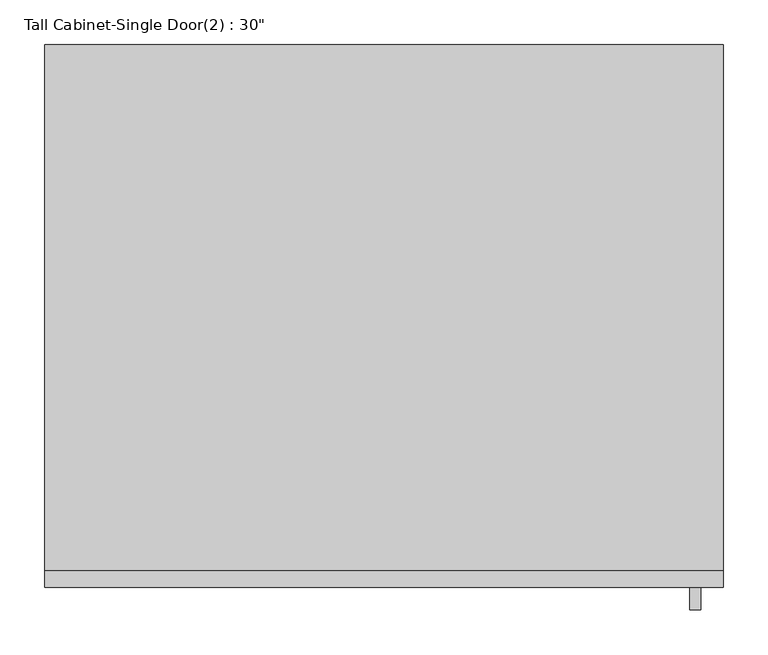
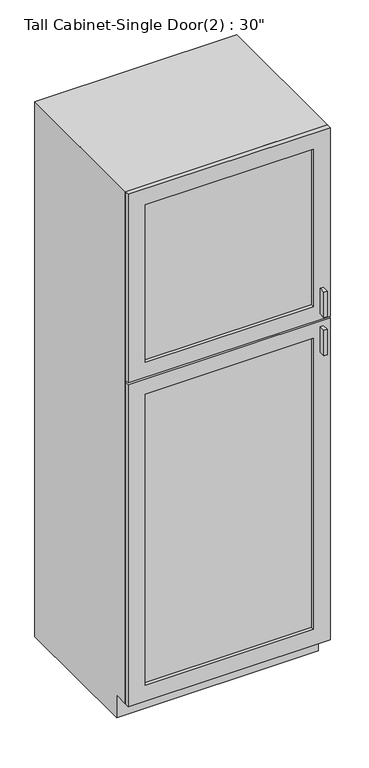
"""IFC4 building model written with IfcOpenShell, lengths in millimetres: furniture geometry."""

from ifc_helpers import new_model, si_unit, frame, origin, place, context, project, spatial, polyline, outline, extrude, faceted_brep, source, transform, mapped, element, save


def furniture_7f1a6afb(model_context):
    return source(origin(), model_context, "Body", "SolidModel", [
        faceted_brep([(399.7377049, -590.55, 90.4875), (399.7377049, -590.55, 2133.6), (-362.2622951, -590.55, 2133.6), (-362.2622951, -590.55, 90.4875), (380.6877049, -590.55, 2114.55), (380.6877049, -590.55, 109.5375), (-343.2122951, -590.55, 109.5375), (-343.2122951, -590.55, 2114.55), (-362.2622951, 0.0, 2133.6), (399.7377049, 0.0, 2133.6), (399.7377049, 0.0, 0.0), (-362.2622951, 0.0, 0.0), (399.7377049, -533.4, 90.4875), (399.7377049, -533.4, 0.0), (-362.2622951, -533.4, 0.0), (-362.2622951, -533.4, 90.4875), (380.6877049, -19.05, 2114.55), (380.6877049, -19.05, 109.5375), (-343.2122951, -19.05, 109.5375), (-343.2122951, -19.05, 2114.55)], [[[0, 1, 2, 3], [4, 5, 6, 7]], [[8, 9, 10, 11]], [[1, 0, 12, 13, 10, 9]], [[2, 1, 9, 8]], [[3, 2, 8, 11, 14, 15]], [[0, 3, 15, 12]], [[5, 4, 16, 17]], [[6, 5, 17, 18]], [[7, 6, 18, 19]], [[4, 7, 19, 16]], [[10, 13, 14, 11]], [[14, 13, 12, 15]], [[17, 16, 19, 18]]]),
        extrude(outline(polyline([(374.3377049, -635.0), (361.8054733, -635.0), (361.8054733, -609.6), (374.3377049, -609.6), (374.3377049, -635.0)])), frame((0.0, 0.0, 1403.5480367), z_axis=(0.0, 0.0, 1.0), x_axis=(1.0, 0.0, 0.0)), (0.0, 0.0, 1.0), 101.6),
        extrude(outline(polyline([(374.3377049, -635.0), (361.8054733, -635.0), (361.8054733, -609.6), (374.3377049, -609.6), (374.3377049, -635.0)])), frame((0.0, 0.0, 1251.1480367), z_axis=(0.0, 0.0, 1.0), x_axis=(1.0, 0.0, 0.0)), (0.0, 0.0, 1.0), 101.6),
        extrude(outline(polyline([(336.2377049, -596.9), (-298.7622951, -596.9), (-298.7622951, -590.55), (336.2377049, -590.55), (336.2377049, -596.9)])), frame((0.0, 0.0, 1441.6480367), z_axis=(0.0, 0.0, 1.0), x_axis=(1.0, 0.0, 0.0)), (0.0, 0.0, 1.0), 628.4519633),
        extrude(outline(polyline([(336.2377049, -596.9), (-298.7622951, -596.9), (-298.7622951, -590.55), (336.2377049, -590.55), (336.2377049, -596.9)])), frame((0.0, 0.0, 153.9875), z_axis=(0.0, 0.0, 1.0), x_axis=(1.0, 0.0, 0.0)), (0.0, 0.0, 1.0), 1160.6605367),
        extrude(outline(polyline([(2133.6, 399.7377049), (2133.6, -362.2622951), (1381.3230367, -362.2622951), (1381.3230367, 399.7377049), (2133.6, 399.7377049)]), holes=[polyline([(2070.1, 336.2377049), (1441.6480367, 336.2377049), (1441.6480367, -298.7622951), (2070.1, -298.7622951), (2070.1, 336.2377049)])]), frame((0.0, -609.6, 0.0), z_axis=(0.0, 1.0, 0.0), x_axis=(0.0, 0.0, 1.0)), (0.0, 0.0, 1.0), 19.05),
        extrude(outline(polyline([(90.4875, 399.7377049), (1374.9730367, 399.7377049), (1374.9730367, -362.2622951), (90.4875, -362.2622951), (90.4875, 399.7377049)]), holes=[polyline([(1314.6480367, 336.2377049), (153.9875, 336.2377049), (153.9875, -298.7622951), (1314.6480367, -298.7622951), (1314.6480367, 336.2377049)])]), frame((0.0, -609.6, 0.0), z_axis=(0.0, 1.0, 0.0), x_axis=(0.0, 0.0, 1.0)), (0.0, 0.0, 1.0), 19.05),
    ])


if __name__ == "__main__":
    model = new_model("IFC4")
    model_context = context("Model", 3, world=origin())
    ifc_project = project(units=[si_unit("LENGTHUNIT", "METRE", prefix="MILLI")], contexts=[model_context])
    site = spatial("IfcSite", under=ifc_project)
    building = spatial("IfcBuilding", under=site)
    placement = place(None, origin())
    furniture_shape = furniture_7f1a6afb(model_context)
    element("IfcFurniture", 1, ObjectType="Tall Cabinet-Single Door(2) : 30\"", at=placement, inside=building, context=model_context, shape_type="MappedRepresentation", body=[
        mapped(furniture_shape, transform((0.0, 0.0, 0.0), x_axis=(1.0, 0.0, 0.0), y_axis=(0.0, 1.0, 0.0), z_axis=(0.0, 0.0, 1.0))),
    ])
    save(model, "model.ifc")

# Revit data of these elements
# Type "Tall Cabinet-Single Door(2) : 30\""
#   Assembly Code = "C1030410"
#   Depth = 2' - 0"
#   Height = 7' - 0"
#   Toe Depth = 0' - 3"
#   Toe Height = 0' - 3 1/2"
#   Width = 2' - 6"
#   Cabinet Material = none
#   Door/Drawer Material = none
#   Handle Material = Cabinets - Handles
#   Panel Material = none
#   Default Elevation = 0
# Element 1 (IfcFurniture, "Tall Cabinet-Single Door(2) : 30\"")
#   Materials on its faces: "Cabinets", "Cabinets - Handles"
# Materials
#   "Cabinets - Handles": class "Metal", colour RGB 57 57 57, transparency 0
#   "Cabinets": colour RGB 249 249 249, transparency 0
